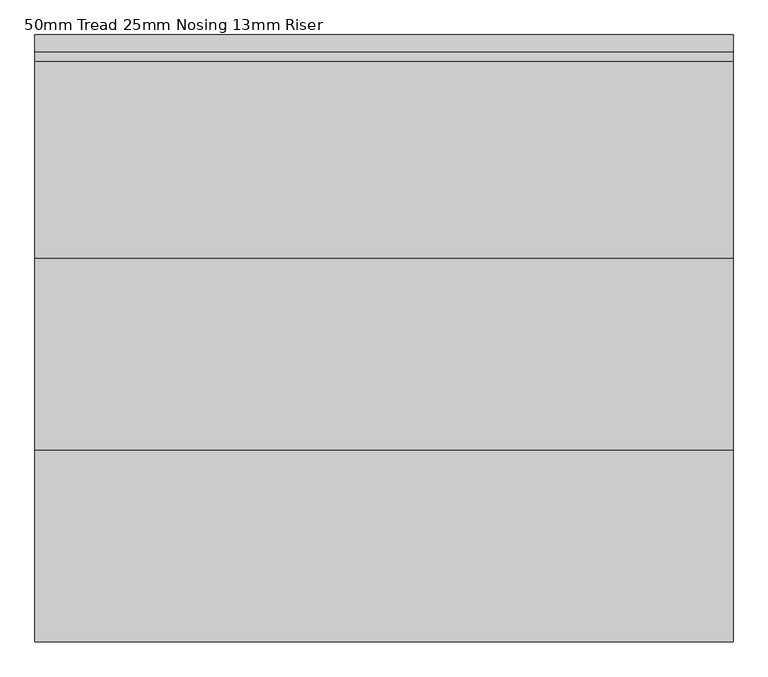
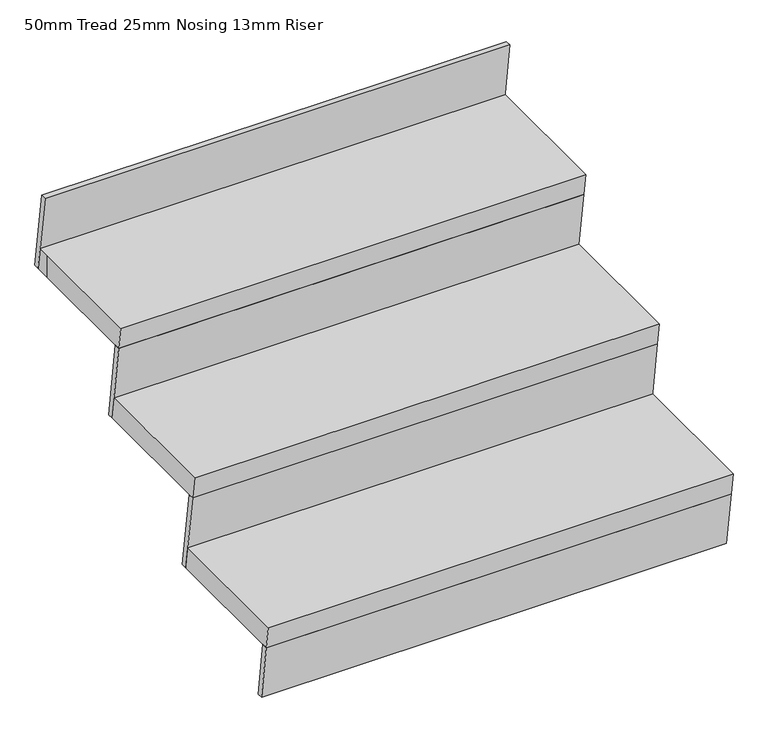
"""IFC4 building model written with IfcOpenShell, lengths in millimetres: stair flight geometry, 50mm Tread 25mm Nosing 13mm Riser."""

from ifc_helpers import new_model, si_unit, origin, place, context, project, spatial, faceted_brep, source, transform, mapped, element, save


def stair_flight_50mm_tread_25mm_nosing_13mm_riser_7e2cbec3(model_context):
    return source(origin(), model_context, "Body", "Brep", [
        faceted_brep([(-9597.1247141, 9297.57664, 173.9130435), (-9597.1247141, 9304.76414, 123.9130435), (-10597.1504953, 9304.76414, 123.9130435), (-10597.1504953, 9297.57664, 173.9130435), (-10597.1504953, 8997.57664, 173.9130435), (-9597.1247141, 8997.57664, 173.9130435), (-9597.1247141, 9004.76414, 123.9130435), (-10597.1504953, 9004.76414, 123.9130435)], [[[0, 1, 2, 3]], [[3, 4, 5, 0]], [[2, 1, 6, 7]], [[4, 3, 2, 7]], [[0, 5, 6, 1]], [[5, 4, 7, 6]]]),
        faceted_brep([(-9597.1247141, 9004.76414, 123.9130435), (-9597.1247141, 9022.57664, 0.0), (-9597.1247141, 9035.20513, 0.0), (-9597.1247141, 9017.39263, 123.9130435), (-10597.1504953, 9004.76414, 123.9130435), (-10597.1504953, 9017.39263, 123.9130435), (-10597.1504953, 9035.20513, 0.0), (-10597.1504953, 9022.57664, 0.0)], [[[0, 1, 2, 3]], [[4, 5, 6, 7]], [[1, 0, 4, 7]], [[2, 1, 7, 6]], [[3, 2, 6, 5]], [[0, 3, 5, 4]]]),
        faceted_brep([(-9597.1247141, 9279.76414, 297.826087), (-9597.1247141, 9304.76414, 123.9130435), (-9597.1247141, 9317.39263, 123.9130435), (-9597.1247141, 9292.39263, 297.826087), (-10597.1504953, 9279.76414, 297.826087), (-10597.1504953, 9292.39263, 297.826087), (-10597.1504953, 9317.39263, 123.9130435), (-10597.1504953, 9304.76414, 123.9130435)], [[[0, 1, 2, 3]], [[4, 5, 6, 7]], [[1, 0, 4, 7]], [[2, 1, 7, 6]], [[3, 2, 6, 5]], [[0, 3, 5, 4]]]),
        faceted_brep([(-10597.1504953, 9572.57664, 347.826087), (-10597.1504953, 9272.57664, 347.826087), (-9597.1247141, 9272.57664, 347.826087), (-9597.1247141, 9572.57664, 347.826087), (-10597.1504953, 9579.76414, 297.826087), (-9597.1247141, 9579.76414, 297.826087), (-9597.1247141, 9279.76414, 297.826087), (-10597.1504953, 9279.76414, 297.826087)], [[[0, 1, 2, 3]], [[4, 5, 6, 7]], [[1, 0, 4, 7]], [[3, 2, 6, 5]], [[3, 5, 4, 0]], [[2, 1, 7, 6]]]),
        faceted_brep([(-9597.1247141, 9829.76414, 645.6521739), (-9597.1247141, 9854.76414, 471.7391304), (-9597.1247141, 9867.39263, 471.7391304), (-9597.1247141, 9842.39263, 645.6521739), (-10597.1504953, 9829.76414, 645.6521739), (-10597.1504953, 9842.39263, 645.6521739), (-10597.1504953, 9867.39263, 471.7391304), (-10597.1504953, 9854.76414, 471.7391304)], [[[0, 1, 2, 3]], [[4, 5, 6, 7]], [[1, 0, 4, 7]], [[2, 1, 7, 6]], [[3, 2, 6, 5]], [[0, 3, 5, 4]]]),
        faceted_brep([(-9597.1247141, 9554.76414, 471.7391304), (-9597.1247141, 9579.76414, 297.826087), (-9597.1247141, 9592.39263, 297.826087), (-9597.1247141, 9567.39263, 471.7391304), (-10597.1504953, 9554.76414, 471.7391304), (-10597.1504953, 9567.39263, 471.7391304), (-10597.1504953, 9592.39263, 297.826087), (-10597.1504953, 9579.76414, 297.826087)], [[[0, 1, 2, 3]], [[4, 5, 6, 7]], [[1, 0, 4, 7]], [[2, 1, 7, 6]], [[3, 2, 6, 5]], [[0, 3, 5, 4]]]),
        faceted_brep([(-10597.1504953, 9847.57664, 521.7391304), (-10597.1504953, 9822.57664, 521.7391304), (-10597.1504953, 9547.57664, 521.7391304), (-9597.1247141, 9547.57664, 521.7391304), (-9597.1247141, 9847.57664, 521.7391304), (-10597.1504953, 9854.76414, 471.7391304), (-9597.1247141, 9854.76414, 471.7391304), (-9597.1247141, 9554.76414, 471.7391304), (-10597.1504953, 9554.76414, 471.7391304), (-10597.1504953, 9822.57664, 471.7391304)], [[[0, 1, 2, 3, 4]], [[5, 6, 7, 8, 9]], [[1, 0, 5, 9]], [[2, 1, 9, 8]], [[4, 3, 7, 6]], [[4, 6, 5, 0]], [[3, 2, 8, 7]]]),
    ])


if __name__ == "__main__":
    model = new_model("IFC4")
    model_context = context("Model", 3, world=origin())
    ifc_project = project(units=[si_unit("LENGTHUNIT", "METRE", prefix="MILLI")], contexts=[model_context])
    site = spatial("IfcSite", under=ifc_project)
    building = spatial("IfcBuilding", under=site)
    placement = place(None, origin())
    stair_flight_50mm_tread_25mm_nosing_13mm_riser_shape = stair_flight_50mm_tread_25mm_nosing_13mm_riser_7e2cbec3(model_context)
    element("IfcStairFlight", 1, ObjectType="50mm Tread 25mm Nosing 13mm Riser", at=placement, inside=building, context=model_context, shape_type="MappedRepresentation", body=[
        mapped(stair_flight_50mm_tread_25mm_nosing_13mm_riser_shape, transform((0.0, 0.0, 0.0), x_axis=(1.0, 0.0, 0.0), y_axis=(0.0, 1.0, 0.0), z_axis=(0.0, 0.0, 1.0))),
    ])
    save(model, "model.ifc")
